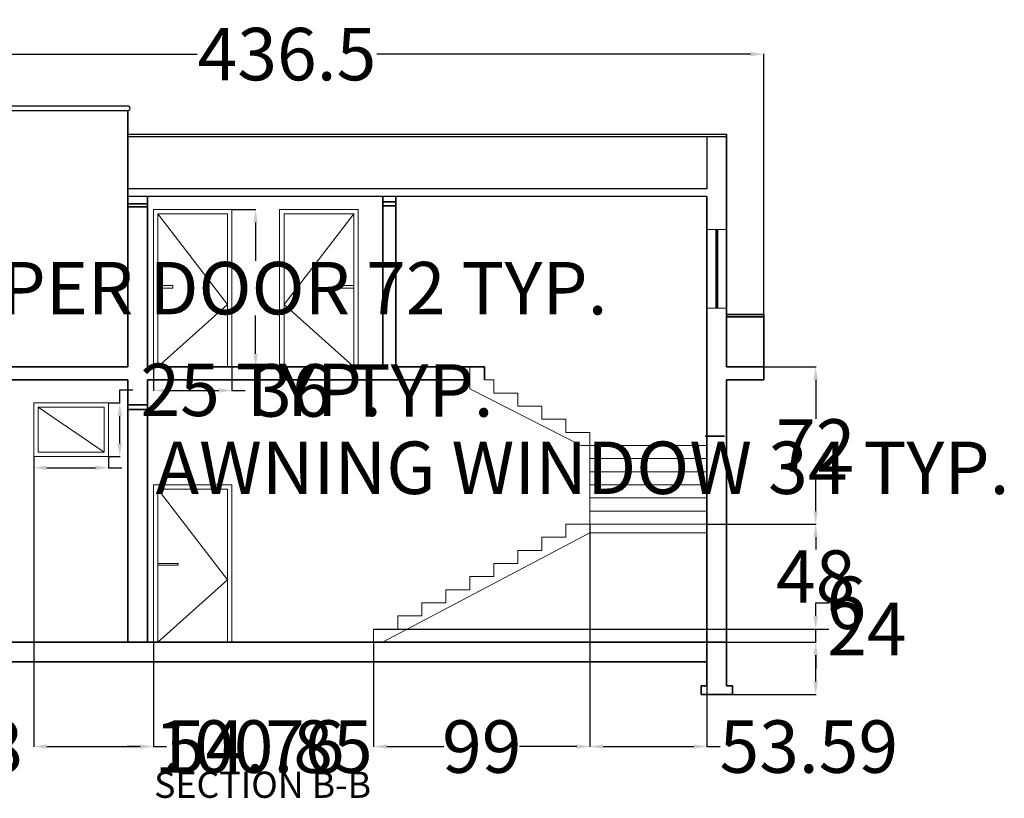
# Model space of a CAD drawing. Units: inches. Extents: x -15 to 1815, y 1023 to 2303.
# Tile 6 of 8: x 1217 to 1668, y 1023 to 1379. Entities that reach past the tile are written whole.
import ezdxf

# ---------------------------------------------------------------- set-up
doc = ezdxf.new("R2010")
doc.units = ezdxf.units.IN
doc.header["$MEASUREMENT"] = 0
for name, color, linetype, lineweight in [('A-ANNO-DIMS', 2, 'Continuous', 18), ('A-ANNO-TEXT', 7, 'Continuous', 25), ('A-DOOR', 3, 'Continuous', 18), ('A-FLOR', 7, 'Continuous', 35), ('A-FLOR-STRS', 3, 'Continuous', 18), ('A-GLAZ', 4, 'Continuous', 18), ('A-ROOF', 7, 'Continuous', 25), ('A-SECT', 7, 'Continuous', 35), ('S-FNDN', 7, 'Continuous', 35)]:
    doc.layers.add(name, color=color, linetype=linetype, lineweight=lineweight)
doc.styles.get("Standard").update_dxf_attribs({"font": 'arial.ttf'})
doc.dimstyles.get("Standard").update_dxf_attribs({"dimtxt": 24, "dimasz": 6, "dimexe": 0.18, "dimexo": 0.0625, "dimgap": 0.09, "dimtad": 0, "dimtih": 1, "dimtoh": 1, "dimdec": 0, "dimzin": 0, "dimdsep": 46, "dimlunit": 3, "dimtxsty": 'Standard', "dimcen": 0.09, "dimadec": 0, "dimazin": 0, "dimtfac": 1, "dimtdec": 0, "dimtofl": 0, "dimtmove": 0, "dimatfit": 3, "dimfxl": 1, "dimtolj": 1, "dimtzin": 0, "dimarcsym": 0})

# ---------------------------------------------------------------- blocks, each defined once
blk = doc.blocks.new('DOOR-36-SEC-LEVER')
for p, q in [((2, 70), (34, 28.45)), ((34, 28.45), (2, 0)), ((2, 2), (2, 0)), ((34, 2), (34, 0))]:
    blk.add_line(p, q)
for points in [[(0, 0), (36, 0), (36, 72), (0, 72)], [(2, 36), (11.36, 36), (11.36, 35.17), (2, 35.17)]]:
    blk.add_lwpolyline(points, close=True)
blk.add_lwpolyline([(34, 2), (34, 70), (2, 70), (2, 2)])
blk = doc.blocks.new('DOOR-36-SEC-RETURN-LEVER')
for p, q in [((2, 70), (34, 28.45)), ((8.91, 37.23), (2, 37.23)), ((8.91, 36), (8.91, 37.23)), ((8.91, 36), (2, 36)), ((34, 28.45), (2, 0)), ((2, 2), (2, 0)), ((34, 2), (34, 0))]:
    blk.add_line(p, q)
for points in [[(0, 0), (36, 0), (36, 72), (0, 72)], [(2, 36), (8.91, 36), (8.91, 36), (2, 36)]]:
    blk.add_lwpolyline(points, close=True)
blk.add_lwpolyline([(34, 2), (34, 70), (2, 70), (2, 2)])
blk = doc.blocks.new('WIN-AWNING-ELEV')
blk.add_line((32.26, 2), (2, 22.53))
for points in [[(0, 24.53), (34.26, 24.53), (34.26, 0), (0, 0)], [(2, 22.53), (32.26, 22.53), (32.26, 2), (2, 2)]]:
    blk.add_lwpolyline(points, close=True)
blk = doc.blocks.new('WIN-36-JAMB-SEC')
for p, q in [((4, 36.04), (4, 0)), ((4.5, 36.04), (4.5, 0)), ((5, 36.04), (5, 0))]:
    blk.add_line(p, q)
blk.add_lwpolyline([(9, 0), (0, 0), (0, 36.04), (9, 36.04)], close=True)
blk = doc.blocks.new('COPING-ROUND-END')
for p, q in [((1.07, 2.13), (126.89, 2.13)), ((1.07, 0), (126.89, 0))]:
    blk.add_line(p, q)
for centre, start, end in [((1.07, 1.07), 90, 270), ((126.89, 1.07), 270, 90)]:
    blk.add_arc(centre, 1.07, start, end)
blk = doc.blocks.new('FOOTING-STRIP-SECTION')
for p, q in [((0, 0), (0, 3.98)), ((0, 3.98), (2.61, 3.98)), ((14.22, 0), (0, 0)), ((14.22, 3.98), (11.61, 3.98)), ((14.22, 0), (14.22, 3.98))]:
    blk.add_line(p, q)
blk = doc.blocks.new('*D51')
at = {"layer": 'A-ANNO-DIMS', "color": 0, "lineweight": -2, "transparency": 16777216}
for p, q in [((1314.04, 1291.99), (1324.95, 1291.99)), ((1324.77, 1285.99), (1324.77, 1268.5)), ((1324.77, 1225.99), (1324.77, 1243.49)), ((1314.04, 1219.99), (1324.95, 1219.99))]:
    blk.add_line(p, q, dxfattribs=at)
at = {"layer": 'A-ANNO-DIMS', "color": 0, "transparency": 16777216}
for points in [[(1323.77, 1285.99), (1325.77, 1285.99), (1324.77, 1291.99)], [(1323.77, 1225.99), (1325.77, 1225.99), (1324.77, 1219.99)]]:
    blk.add_solid(points, dxfattribs=at)
at = {"layer": 'Defpoints', "color": 0, "transparency": 16777216}
for p in [(1313.97, 1291.99), (1324.77, 1291.99), (1313.97, 1219.99)]:
    blk.add_point(p, dxfattribs=at)
at = {"layer": 'A-ANNO-DIMS', "color": 0, "transparency": 16777216, "insert": (1324.77, 1255.99), "char_height": 24, "attachment_point": 5}
blk.add_mtext('\\A1;UPPER DOOR 72 TYP.', dxfattribs=at)
blk = doc.blocks.new('*D52')
at = {"layer": 'A-ANNO-DIMS', "color": 0, "lineweight": -2, "transparency": 16777216}
for p, q in [((1277.97, 1219.93), (1277.97, 1209.01)), ((1313.97, 1219.93), (1313.97, 1209.01)), ((1283.97, 1209.19), (1307.97, 1209.19)), ((1313.97, 1209.19), (1319.97, 1209.19))]:
    blk.add_line(p, q, dxfattribs=at)
at = {"layer": 'A-ANNO-DIMS', "color": 0, "transparency": 16777216}
for points in [[(1283.97, 1210.19), (1283.97, 1208.19), (1277.97, 1209.19)], [(1307.97, 1210.19), (1307.97, 1208.19), (1313.97, 1209.19)]]:
    blk.add_solid(points, dxfattribs=at)
at = {"layer": 'Defpoints', "color": 0, "transparency": 16777216}
for p in [(1277.97, 1219.99), (1313.97, 1219.99), (1313.97, 1209.19)]:
    blk.add_point(p, dxfattribs=at)
at = {"layer": 'A-ANNO-DIMS', "color": 0, "transparency": 16777216, "insert": (1378.47, 1209.19), "char_height": 24, "attachment_point": 5}
blk.add_mtext('\\A1;36 TYP.', dxfattribs=at)
blk = doc.blocks.new('*D53')
at = {"layer": 'A-ANNO-DIMS', "color": 0, "lineweight": -2, "transparency": 16777216}
for p, q in [((1223.21, 1178.86), (1223.21, 1173.61)), ((1257.47, 1178.86), (1257.47, 1173.61)), ((1229.21, 1173.79), (1251.47, 1173.79)), ((1257.47, 1173.79), (1263.47, 1173.79))]:
    blk.add_line(p, q, dxfattribs=at)
at = {"layer": 'A-ANNO-DIMS', "color": 0, "transparency": 16777216}
for points in [[(1229.21, 1174.79), (1229.21, 1172.79), (1223.21, 1173.79)], [(1251.47, 1174.79), (1251.47, 1172.79), (1257.47, 1173.79)]]:
    blk.add_solid(points, dxfattribs=at)
at = {"layer": 'Defpoints', "color": 0, "transparency": 16777216}
for p in [(1223.21, 1178.93), (1257.47, 1178.93), (1257.47, 1173.79)]:
    blk.add_point(p, dxfattribs=at)
at = {"layer": 'A-ANNO-DIMS', "color": 0, "transparency": 16777216, "insert": (1474.45, 1173.79), "char_height": 24, "attachment_point": 5}
blk.add_mtext('\\A1;AWNING WINDOW 34 TYP.', dxfattribs=at)
blk = doc.blocks.new('*D54')
at = {"layer": 'A-ANNO-DIMS', "color": 0, "lineweight": -2, "transparency": 16777216}
for p, q in [((1262.6, 1203.46), (1262.6, 1209.46)), ((1262.6, 1209.46), (1268.6, 1209.46)), ((1257.53, 1203.46), (1262.78, 1203.46)), ((1262.6, 1184.93), (1262.6, 1197.46)), ((1257.53, 1178.93), (1262.78, 1178.93))]:
    blk.add_line(p, q, dxfattribs=at)
at = {"layer": 'A-ANNO-DIMS', "color": 0, "transparency": 16777216}
for points in [[(1261.6, 1197.46), (1263.6, 1197.46), (1262.6, 1203.46)], [(1261.6, 1184.93), (1263.6, 1184.93), (1262.6, 1178.93)]]:
    blk.add_solid(points, dxfattribs=at)
at = {"layer": 'Defpoints', "color": 0, "transparency": 16777216}
for p in [(1257.47, 1203.46), (1262.6, 1203.46), (1257.47, 1178.93)]:
    blk.add_point(p, dxfattribs=at)
at = {"layer": 'A-ANNO-DIMS', "color": 0, "transparency": 16777216, "insert": (1327.31, 1209.46), "char_height": 24, "attachment_point": 5}
blk.add_mtext('\\A1;25 TYP.', dxfattribs=at)
blk = doc.blocks.new('*D113')
at = {"layer": 'A-ANNO-DIMS', "color": 0, "lineweight": -2, "transparency": 16777216}
for p, q in [((1120.86, 1244.06), (1120.86, 1363.3)), ((1126.86, 1363.12), (1297.96, 1363.12)), ((1551.37, 1363.12), (1380.27, 1363.12)), ((1557.37, 1244.06), (1557.37, 1363.3))]:
    blk.add_line(p, q, dxfattribs=at)
at = {"layer": 'A-ANNO-DIMS', "color": 0, "transparency": 16777216}
for points in [[(1126.86, 1364.12), (1126.86, 1362.12), (1120.86, 1363.12)], [(1551.37, 1364.12), (1551.37, 1362.12), (1557.37, 1363.12)]]:
    blk.add_solid(points, dxfattribs=at)
at = {"layer": 'Defpoints', "color": 0, "transparency": 16777216}
for p in [(1557.37, 1363.12), (1120.86, 1243.99), (1557.37, 1243.99)]:
    blk.add_point(p, dxfattribs=at)
at = {"layer": 'A-ANNO-DIMS', "color": 0, "transparency": 16777216, "insert": (1339.12, 1363.12), "char_height": 24, "attachment_point": 5}
blk.add_mtext('\\A1;436.5', dxfattribs=at)
blk = doc.blocks.new('*D115')
at = {"layer": 'A-ANNO-DIMS', "color": 0, "lineweight": -2, "transparency": 16777216}
for p, q in [((1581.17, 1093.99), (1581.17, 1099.99)), ((1581.17, 1099.99), (1587.17, 1099.99)), ((1540.47, 1093.99), (1581.35, 1093.99)), ((1581.17, 1075.99), (1581.17, 1087.99)), ((1543.08, 1069.99), (1581.35, 1069.99))]:
    blk.add_line(p, q, dxfattribs=at)
at = {"layer": 'A-ANNO-DIMS', "color": 0, "transparency": 16777216}
for points in [[(1580.17, 1087.99), (1582.17, 1087.99), (1581.17, 1093.99)], [(1580.17, 1075.99), (1582.17, 1075.99), (1581.17, 1069.99)]]:
    blk.add_solid(points, dxfattribs=at)
at = {"layer": 'Defpoints', "color": 0, "transparency": 16777216}
for p in [(1540.41, 1093.99), (1581.17, 1093.99), (1543.02, 1069.99)]:
    blk.add_point(p, dxfattribs=at)
at = {"layer": 'A-ANNO-DIMS', "color": 0, "transparency": 16777216, "insert": (1604.6, 1099.99), "char_height": 24, "attachment_point": 5}
blk.add_mtext('\\A1;24', dxfattribs=at)
blk = doc.blocks.new('*D116')
at = {"layer": 'A-ANNO-DIMS', "color": 0, "lineweight": -2, "transparency": 16777216}
for p, q in [((1581.17, 1105.99), (1581.17, 1111.99)), ((1581.17, 1111.99), (1587.17, 1111.99)), ((1378.88, 1099.99), (1581.35, 1099.99)), ((1378.88, 1093.99), (1581.35, 1093.99)), ((1581.17, 1087.99), (1581.17, 1081.99))]:
    blk.add_line(p, q, dxfattribs=at)
at = {"layer": 'A-ANNO-DIMS', "color": 0, "transparency": 16777216}
for points in [[(1580.17, 1105.99), (1582.17, 1105.99), (1581.17, 1099.99)], [(1580.17, 1087.99), (1582.17, 1087.99), (1581.17, 1093.99)]]:
    blk.add_solid(points, dxfattribs=at)
at = {"layer": 'Defpoints', "color": 0, "transparency": 16777216}
for p in [(1378.82, 1099.99), (1581.17, 1099.99), (1378.82, 1093.99)]:
    blk.add_point(p, dxfattribs=at)
at = {"layer": 'A-ANNO-DIMS', "color": 0, "transparency": 16777216, "insert": (1595.18, 1111.99), "char_height": 24, "attachment_point": 5}
blk.add_mtext('\\A1;6', dxfattribs=at)
blk = doc.blocks.new('*D117')
at = {"layer": 'A-ANNO-DIMS', "color": 0, "lineweight": -2, "transparency": 16777216}
for p, q in [((1531.47, 1147.99), (1581.35, 1147.99)), ((1581.17, 1141.99), (1581.17, 1136.34)), ((1581.17, 1105.99), (1581.17, 1111.65)), ((1378.88, 1099.99), (1581.35, 1099.99))]:
    blk.add_line(p, q, dxfattribs=at)
at = {"layer": 'A-ANNO-DIMS', "color": 0, "transparency": 16777216}
for points in [[(1580.17, 1141.99), (1582.17, 1141.99), (1581.17, 1147.99)], [(1580.17, 1105.99), (1582.17, 1105.99), (1581.17, 1099.99)]]:
    blk.add_solid(points, dxfattribs=at)
at = {"layer": 'Defpoints', "color": 0, "transparency": 16777216}
for p in [(1531.41, 1147.99), (1581.17, 1147.99), (1378.82, 1099.99)]:
    blk.add_point(p, dxfattribs=at)
at = {"layer": 'A-ANNO-DIMS', "color": 0, "transparency": 16777216, "insert": (1581.17, 1123.99), "char_height": 24, "attachment_point": 5}
blk.add_mtext('\\A1;48', dxfattribs=at)
blk = doc.blocks.new('*D118')
at = {"layer": 'A-ANNO-DIMS', "color": 0, "lineweight": -2, "transparency": 16777216}
for p, q in [((1557.43, 1219.99), (1581.35, 1219.99)), ((1581.17, 1213.99), (1581.17, 1196.13)), ((1581.17, 1153.99), (1581.17, 1171.86)), ((1531.47, 1147.99), (1581.35, 1147.99))]:
    blk.add_line(p, q, dxfattribs=at)
at = {"layer": 'A-ANNO-DIMS', "color": 0, "transparency": 16777216}
for points in [[(1580.17, 1213.99), (1582.17, 1213.99), (1581.17, 1219.99)], [(1580.17, 1153.99), (1582.17, 1153.99), (1581.17, 1147.99)]]:
    blk.add_solid(points, dxfattribs=at)
at = {"layer": 'Defpoints', "color": 0, "transparency": 16777216}
for p in [(1557.37, 1219.99), (1581.17, 1219.99), (1531.41, 1147.99)]:
    blk.add_point(p, dxfattribs=at)
at = {"layer": 'A-ANNO-DIMS', "color": 0, "transparency": 16777216, "insert": (1581.17, 1183.99), "char_height": 24, "attachment_point": 5}
blk.add_mtext('\\A1;72', dxfattribs=at)
blk = doc.blocks.new('*D119')
at = {"layer": 'A-ANNO-DIMS', "color": 0, "lineweight": -2, "transparency": 16777216}
for p, q in [((1223.21, 1178.86), (1223.21, 1046.01)), ((1149.41, 1093.93), (1149.41, 1046.01)), ((1143.41, 1046.19), (1137.41, 1046.19)), ((1229.21, 1046.19), (1235.21, 1046.19))]:
    blk.add_line(p, q, dxfattribs=at)
at = {"layer": 'A-ANNO-DIMS', "color": 0, "transparency": 16777216}
for points in [[(1143.41, 1047.19), (1143.41, 1045.19), (1149.41, 1046.19)], [(1229.21, 1047.19), (1229.21, 1045.19), (1223.21, 1046.19)]]:
    blk.add_solid(points, dxfattribs=at)
at = {"layer": 'Defpoints', "color": 0, "transparency": 16777216}
for p in [(1223.21, 1178.93), (1149.41, 1093.99), (1223.21, 1046.19)]:
    blk.add_point(p, dxfattribs=at)
at = {"layer": 'A-ANNO-DIMS', "color": 0, "transparency": 16777216, "insert": (1186.31, 1046.19), "char_height": 24, "attachment_point": 5}
blk.add_mtext('\\A1;73.8', dxfattribs=at)
blk = doc.blocks.new('*D120')
at = {"layer": 'A-ANNO-DIMS', "color": 0, "lineweight": -2, "transparency": 16777216}
for p, q in [((1223.21, 1178.86), (1223.21, 1046.01)), ((1277.97, 1093.93), (1277.97, 1046.01)), ((1229.21, 1046.19), (1271.97, 1046.19)), ((1277.97, 1046.19), (1283.97, 1046.19))]:
    blk.add_line(p, q, dxfattribs=at)
at = {"layer": 'A-ANNO-DIMS', "color": 0, "transparency": 16777216}
for points in [[(1229.21, 1047.19), (1229.21, 1045.19), (1223.21, 1046.19)], [(1271.97, 1047.19), (1271.97, 1045.19), (1277.97, 1046.19)]]:
    blk.add_solid(points, dxfattribs=at)
at = {"layer": 'Defpoints', "color": 0, "transparency": 16777216}
for p in [(1223.21, 1178.93), (1277.97, 1093.99), (1277.97, 1046.19)]:
    blk.add_point(p, dxfattribs=at)
at = {"layer": 'A-ANNO-DIMS', "color": 0, "transparency": 16777216, "insert": (1324.55, 1046.19), "char_height": 24, "attachment_point": 5}
blk.add_mtext('\\A1;54.76', dxfattribs=at)
blk = doc.blocks.new('*D121')
at = {"layer": 'A-ANNO-DIMS', "color": 0, "lineweight": -2, "transparency": 16777216}
for p, q in [((1277.973923, 1093.932183), (1277.973923, 1046.014683)), ((1378.822077, 1093.932183), (1378.822077, 1046.014683)), ((1271.973923, 1046.194683), (1265.973923, 1046.194683)), ((1384.822077, 1046.194683), (1390.822077, 1046.194683))]:
    blk.add_line(p, q, dxfattribs=at)
at = {"layer": 'A-ANNO-DIMS', "color": 0, "transparency": 16777216}
for points in [[(1271.973923, 1047.194683), (1271.973923, 1045.194683), (1277.973923, 1046.194683)], [(1384.822077, 1047.194683), (1384.822077, 1045.194683), (1378.822077, 1046.194683)]]:
    blk.add_solid(points, dxfattribs=at)
at = {"layer": 'Defpoints', "color": 0, "transparency": 16777216}
for p in [(1277.973923, 1093.994683), (1378.822077, 1093.994683), (1378.822077, 1046.194683)]:
    blk.add_point(p, dxfattribs=at)
at = {"layer": 'A-ANNO-DIMS', "color": 0, "transparency": 16777216, "insert": (1328.398, 1046.194683), "char_height": 24, "attachment_point": 5}
blk.add_mtext('\\A1;100.85', dxfattribs=at)
blk = doc.blocks.new('*D122')
at = {"layer": 'A-ANNO-DIMS', "color": 0, "lineweight": -2, "transparency": 16777216}
for p, q in [((1477.82, 1147.93), (1477.82, 1046.01)), ((1378.82, 1093.93), (1378.82, 1046.01)), ((1384.82, 1046.19), (1411.02, 1046.19)), ((1471.82, 1046.19), (1445.63, 1046.19))]:
    blk.add_line(p, q, dxfattribs=at)
at = {"layer": 'A-ANNO-DIMS', "color": 0, "transparency": 16777216}
for points in [[(1384.82, 1047.19), (1384.82, 1045.19), (1378.82, 1046.19)], [(1471.82, 1047.19), (1471.82, 1045.19), (1477.82, 1046.19)]]:
    blk.add_solid(points, dxfattribs=at)
at = {"layer": 'Defpoints', "color": 0, "transparency": 16777216}
for p in [(1477.82, 1147.99), (1378.82, 1093.99), (1477.82, 1046.19)]:
    blk.add_point(p, dxfattribs=at)
at = {"layer": 'A-ANNO-DIMS', "color": 0, "transparency": 16777216, "insert": (1428.32, 1046.19), "char_height": 24, "attachment_point": 5}
blk.add_mtext('\\A1;99', dxfattribs=at)
blk = doc.blocks.new('*D123')
at = {"layer": 'A-ANNO-DIMS', "color": 0, "lineweight": -2, "transparency": 16777216}
for p, q in [((1477.82, 1147.93), (1477.82, 1046.01)), ((1531.41, 1147.93), (1531.41, 1046.01)), ((1483.82, 1046.19), (1525.41, 1046.19)), ((1531.41, 1046.19), (1537.41, 1046.19))]:
    blk.add_line(p, q, dxfattribs=at)
at = {"layer": 'A-ANNO-DIMS', "color": 0, "transparency": 16777216}
for points in [[(1483.82, 1047.19), (1483.82, 1045.19), (1477.82, 1046.19)], [(1525.41, 1047.19), (1525.41, 1045.19), (1531.41, 1046.19)]]:
    blk.add_solid(points, dxfattribs=at)
at = {"layer": 'Defpoints', "color": 0, "transparency": 16777216}
for p in [(1477.82, 1147.99), (1531.41, 1147.99), (1531.41, 1046.19)]:
    blk.add_point(p, dxfattribs=at)
at = {"layer": 'A-ANNO-DIMS', "color": 0, "transparency": 16777216, "insert": (1578.02, 1046.19), "char_height": 24, "attachment_point": 5}
blk.add_mtext('\\A1;53.59', dxfattribs=at)

msp = doc.modelspace()

# ---------------------------------------------------------------- linework, layer by layer
at = {"layer": 'A-FLOR'}
for p, q in [((1557.3693, 1243.9947), (1540.4077, 1243.9947)), ((1557.3693, 1243.9947), (1540.4077, 1243.9947)), ((1557.3693, 1242.8854), (1540.4077, 1242.8854)), ((1557.3693, 1243.9947), (1557.3693, 1213.9947)), ((1266.2321, 1219.9947), (1140.4077, 1219.9947)), ((1382.9528, 1219.9947), (1275.2321, 1219.9947)), ((1429.568, 1219.9947), (1388.9528, 1219.9947)), ((1429.568, 1219.9947), (1429.568, 1213.9947)), ((1557.3693, 1219.9947), (1540.4077, 1219.9947)), ((1266.2321, 1213.9947), (1140.4077, 1213.9947)), ((1422.8221, 1213.9947), (1275.2321, 1213.9947)), ((1557.3693, 1213.9947), (1540.4077, 1213.9947)), ((1266.2321, 1093.9947), (1140.4077, 1093.9947)), ((1540.4077, 1093.9947), (1266.2321, 1093.9947)), ((1266.2321, 1084.9947), (1149.4077, 1084.9947)), ((1531.4077, 1084.9947), (1266.2321, 1084.9947))]:
    msp.add_line(p, q, dxfattribs=at)
at = {"layer": 'A-FLOR-STRS'}
for p, q in [((1422.8221, 1219.9947), (1411.8221, 1219.9947)), ((1422.8221, 1213.9947), (1422.8221, 1219.9947)), ((1422.8221, 1213.9947), (1422.8221, 1209.9947)), ((1433.8221, 1213.9947), (1429.568, 1213.9947)), ((1433.8221, 1207.9947), (1433.8221, 1213.9947)), ((1473.8221, 1183.9947), (1422.8221, 1209.9947)), ((1444.8221, 1207.9947), (1433.8221, 1207.9947)), ((1444.8221, 1201.9947), (1444.8221, 1207.9947)), ((1455.8221, 1201.9947), (1444.8221, 1201.9947)), ((1455.8221, 1195.9947), (1455.8221, 1201.9947)), ((1466.8221, 1195.9947), (1455.8221, 1195.9947)), ((1466.8221, 1189.9947), (1466.8221, 1195.9947)), ((1477.8221, 1189.9947), (1466.8221, 1189.9947)), ((1477.8221, 1183.9947), (1477.8221, 1189.9947)), ((1477.8221, 1183.9947), (1473.8221, 1183.9947)), ((1477.8221, 1183.9947), (1531.4077, 1183.9947)), ((1477.8221, 1147.9947), (1477.8221, 1183.9947)), ((1477.8221, 1177.9947), (1531.4077, 1177.9947)), ((1477.8221, 1171.9947), (1531.4077, 1171.9947)), ((1477.8221, 1165.9947), (1531.4077, 1165.9947)), ((1477.8221, 1159.9947), (1531.4077, 1159.9947)), ((1477.8221, 1153.9947), (1531.4077, 1153.9947)), ((1466.8221, 1141.9947), (1466.8221, 1147.9947)), ((1466.8221, 1147.9947), (1477.8221, 1147.9947)), ((1477.8221, 1147.9947), (1531.4077, 1147.9947)), ((1477.8221, 1143.9947), (1382.8221, 1093.9947)), ((1455.8221, 1135.9947), (1455.8221, 1141.9947)), ((1455.8221, 1141.9947), (1466.8221, 1141.9947)), ((1477.8221, 1143.9947), (1531.4077, 1143.9947)), ((1444.8221, 1129.9947), (1444.8221, 1135.9947)), ((1444.8221, 1135.9947), (1455.8221, 1135.9947)), ((1433.8221, 1123.9947), (1433.8221, 1129.9947)), ((1433.8221, 1129.9947), (1444.8221, 1129.9947)), ((1422.8221, 1117.9947), (1422.8221, 1123.9947)), ((1422.8221, 1123.9947), (1433.8221, 1123.9947)), ((1411.8221, 1111.9947), (1411.8221, 1117.9947)), ((1411.8221, 1117.9947), (1422.8221, 1117.9947)), ((1400.8221, 1105.9947), (1400.8221, 1111.9947)), ((1400.8221, 1111.9947), (1411.8221, 1111.9947)), ((1389.8221, 1099.9947), (1389.8221, 1105.9947)), ((1389.8221, 1105.9947), (1400.8221, 1105.9947)), ((1378.8221, 1093.9947), (1378.8221, 1099.9947)), ((1378.8221, 1099.9947), (1389.8221, 1099.9947)), ((1378.8221, 1093.9947), (1382.8221, 1093.9947))]:
    msp.add_line(p, q, dxfattribs=at)
at = {"layer": 'A-ROOF'}
for p, q in [((1540.41, 1326.3315), (1266.2345, 1326.3315)), ((1540.41, 1325.2295), (1266.2345, 1325.2295)), ((1531.4077, 1325.2295), (1531.4077, 1301.5252)), ((1531.4077, 1301.5252), (1266.2321, 1301.5252)), ((1531.4077, 1297.9947), (1266.2321, 1297.9947))]:
    msp.add_line(p, q, dxfattribs=at)
at = {"layer": 'A-SECT'}
for p, q in [((1266.2321, 1297.9947), (1266.2321, 1337.1888)), ((1540.4077, 1326.3315), (1540.4077, 1219.9947)), ((1266.2321, 1297.9947), (1266.2321, 1219.9947)), ((1275.2321, 1297.9947), (1275.2321, 1219.9947)), ((1382.9528, 1297.9947), (1382.9528, 1219.9947)), ((1388.9528, 1297.9947), (1388.9528, 1219.9947)), ((1531.4077, 1297.9947), (1531.4077, 1194.7455)), ((1266.2321, 1213.9947), (1266.2321, 1093.9947)), ((1275.2321, 1213.9947), (1275.2321, 1093.9947)), ((1540.4077, 1213.9947), (1540.4077, 1194.7455)), ((1531.4077, 1194.7455), (1531.4077, 1093.9947)), ((1540.4077, 1194.7455), (1540.4077, 1093.9947)), ((1530.4997, 1188.3197), (1539.4997, 1188.3197))]:
    msp.add_line(p, q, dxfattribs=at)
for points in [[(1266.2321, 1294.5817), (1275.2321, 1294.5817), (1275.2321, 1293.2159), (1266.2321, 1293.2159)], [(1382.9528, 1295.5592), (1388.9528, 1295.5592), (1388.9528, 1293.6193), (1382.9528, 1293.6193)], [(1266.2321, 1202.6306), (1275.2321, 1202.6306), (1275.2321, 1200.4591), (1266.2321, 1200.4591)]]:
    msp.add_lwpolyline(points, close=True, dxfattribs=at)
at = {"layer": 'S-FNDN'}
for p, q in [((1531.4077, 1169.5723), (1531.4077, 1073.9782)), ((1531.4077, 1169.5723), (1531.4077, 1073.9782)), ((1540.4077, 1169.5723), (1540.4077, 1073.9782)), ((1540.4077, 1069.9947), (1528.7975, 1069.9947))]:
    msp.add_line(p, q, dxfattribs=at)

# ---------------------------------------------------------------- block references
at = {"layer": 'A-DOOR'}
for name, p in [('DOOR-36-SEC-RETURN-LEVER', (1277.9739, 1219.9947)), ('DOOR-36-SEC-LEVER', (1277.9739, 1093.9947))]:
    msp.add_blockref(name, p, dxfattribs=at)
at = {"layer": 'A-DOOR', "extrusion": (0, 0, -1), "zscale": -1}
msp.add_blockref('DOOR-36-SEC-RETURN-LEVER', (-1371.7843, 1219.9947), dxfattribs=at)
at = {"layer": 'A-GLAZ'}
for name, p in [('WIN-36-JAMB-SEC', (1531.4077, 1246.7648)), ('WIN-AWNING-ELEV', (1223.2102, 1178.9271))]:
    msp.add_blockref(name, p, dxfattribs=at)
at = {"layer": 'A-ROOF', "rotation": 180}
msp.add_blockref('COPING-ROUND-END', (1267.298, 1339.3206), dxfattribs=at)
at = {"layer": 'S-FNDN'}
msp.add_blockref('FOOTING-STRIP-SECTION', (1528.7975, 1069.9947), dxfattribs=at)

# ---------------------------------------------------------------- texts
at = {"layer": 'A-ANNO-TEXT'}
msp.add_text('SECTION B-B', height=12, dxfattribs=at).set_placement((1278.3397, 1022.7252))

# ---------------------------------------------------------------- dimensions: what is measured, and where the dimension line sits
at = {"layer": 'A-ANNO-DIMS'}
for base, p1, p2, override, picture, middle in [((1557.3693, 1363.1206), (1120.864, 1243.9947), (1557.3693, 1243.9947), {"dimdec": 1, "dimlfac": 1, "dimrnd": 0, "dimzin": 0, "dimdsep": 46, "dimlunit": 2}, '*D113', (1339.1166, 1363.1206)), ((1223.2102, 1046.1947), (1149.4077, 1093.9947), (1223.2102, 1178.9271), {"dimdec": 1, "dimlfac": 1, "dimrnd": 0, "dimzin": 0, "dimdsep": 46, "dimlunit": 2}, '*D119', (1186.309, 1046.1947)), ((1277.9739, 1046.1947), (1223.2102, 1178.9271), (1277.9739, 1093.9947), {"dimdec": 2, "dimlfac": 1, "dimrnd": 0, "dimzin": 0, "dimdsep": 46, "dimlunit": 2}, '*D120', (1324.5496, 1046.1947)), ((1477.8221, 1046.1947), (1378.8221, 1093.9947), (1477.8221, 1147.9947), {"dimdec": 0, "dimlfac": 1, "dimrnd": 0, "dimzin": 0, "dimdsep": 46, "dimlunit": 2}, '*D122', (1428.3221, 1046.1947)), ((1531.4077, 1046.1947), (1477.8221, 1147.9947), (1531.4077, 1147.9947), {"dimdec": 2, "dimlfac": 1, "dimrnd": 0, "dimzin": 0, "dimdsep": 46, "dimlunit": 2}, '*D123', (1578.0161, 1046.1947)), ((1378.8221, 1046.1947), (1277.9739, 1093.9947), (1378.8221, 1093.9947), {"dimdec": 2, "dimlfac": 1, "dimrnd": 0, "dimzin": 0, "dimdsep": 46, "dimlunit": 2}, '*D121', (1328.398, 1046.1947))]:
    dim = msp.add_linear_dim(base=base, p1=p1, p2=p2, dimstyle='Standard', override=override, dxfattribs=at)
    dim.commit()
    dim.dimension.update_dxf_attribs({"geometry": picture, "text_midpoint": middle})
for base, p1, p2, text, picture, middle in [((1324.7739, 1291.9947), (1313.9739, 1219.9947), (1313.9739, 1291.9947), 'UPPER DOOR <> TYP.', '*D51', (1324.7739, 1255.9947)), ((1262.6039, 1203.4553), (1257.4656, 1178.9271), (1257.4656, 1203.4553), '<> TYP.', '*D54', (1327.3105, 1209.4553))]:
    dim = msp.add_linear_dim(base=base, p1=p1, p2=p2, angle=90, text=text, dimstyle='Standard', override={"dimdec": 0, "dimlfac": 1, "dimrnd": 0, "dimzin": 0, "dimdsep": 46, "dimlunit": 2}, dxfattribs=at)
    dim.commit()
    dim.dimension.update_dxf_attribs({"geometry": picture, "text_midpoint": middle})
for base, p1, p2, text, picture, middle in [((1257.4656, 1173.7888), (1223.2102, 1178.9271), (1257.4656, 1178.9271), 'AWNING WINDOW <> TYP.', '*D53', (1474.4478, 1173.7888)), ((1313.9739, 1209.1947), (1277.9739, 1219.9947), (1313.9739, 1219.9947), '<> TYP.', '*D52', (1378.4677, 1209.1947))]:
    dim = msp.add_linear_dim(base=base, p1=p1, p2=p2, text=text, dimstyle='Standard', override={"dimdec": 0, "dimlfac": 1, "dimrnd": 0, "dimzin": 0, "dimdsep": 46, "dimlunit": 2}, dxfattribs=at)
    dim.commit()
    dim.dimension.update_dxf_attribs({"geometry": picture, "text_midpoint": middle})
for base, p1, p2, picture, middle in [((1581.1693, 1219.9947), (1531.4077, 1147.9947), (1557.3693, 1219.9947), '*D118', (1581.1693, 1183.9947)), ((1581.1693, 1147.9947), (1378.8221, 1099.9947), (1531.4077, 1147.9947), '*D117', (1581.1693, 1123.9947)), ((1581.1693, 1099.9947), (1378.8221, 1093.9947), (1378.8221, 1099.9947), '*D116', (1595.1829, 1111.9947)), ((1581.1693, 1093.9947), (1543.0178, 1069.9947), (1540.4077, 1093.9947), '*D115', (1604.6045, 1099.9947))]:
    dim = msp.add_linear_dim(base=base, p1=p1, p2=p2, angle=90, dimstyle='Standard', override={"dimdec": 0, "dimlfac": 1, "dimrnd": 0, "dimzin": 0, "dimdsep": 46, "dimlunit": 2}, dxfattribs=at)
    dim.commit()
    dim.dimension.update_dxf_attribs({"geometry": picture, "text_midpoint": middle})

doc.saveas('drawing.dxf')
